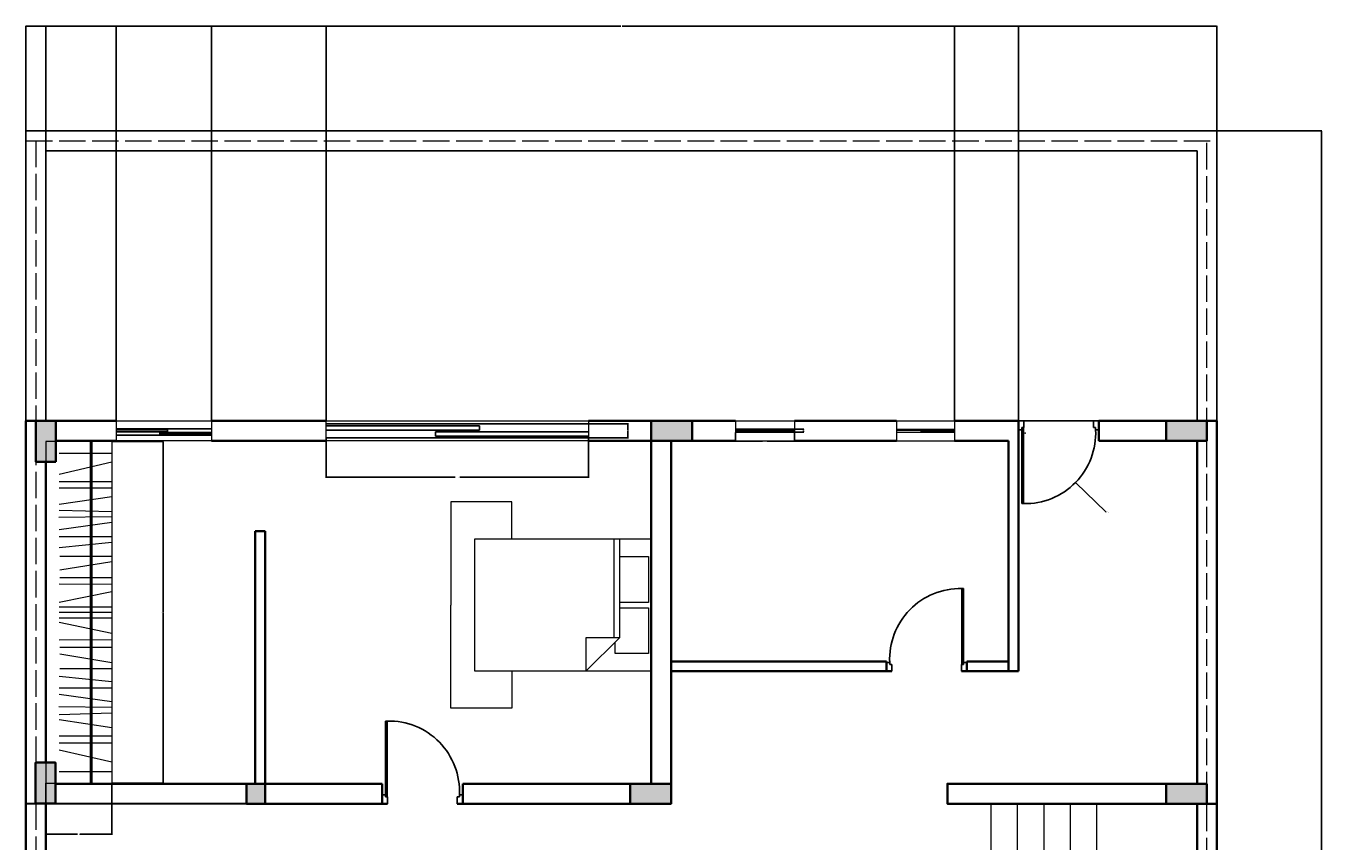
# Model space of a CAD drawing. Units: inches. Extents: x 2711 to 4246, y 540 to 1583.
# Tile 7 of 7: x 3658 to 4246, y 1213 to 1583. Entities that reach past the tile are written whole.
import ezdxf

# ---------------------------------------------------------------- set-up
doc = ezdxf.new("R2010")
doc.units = ezdxf.units.IN
doc.linetypes.add('ACAD_ISO02W100', pattern=[15, 12, -3])
for name, color, linetype, lineweight in [('A-ANNO-DIMS', 2, 'Continuous', 18), ('A-COLS', 210, 'Continuous', 35), ('A-COLS-PATT', 6, 'Continuous', 13), ('A-FLOR-CASE', 30, 'Continuous', 18), ('A-FLOR-STRS', 4, 'Continuous', 18), ('A-GLAZ', 4, 'Continuous', 18), ('A-WALL', 1, 'Continuous', 35), ('C-PROP-HIDN', 7, 'ACAD_ISO02W100', 13), ('C-PROP-WALL', 7, 'Continuous', 25), ('DOOR', 32, 'Continuous', 25), ('FURN', 30, 'Continuous', 18)]:
    doc.layers.add(name, color=color, linetype=linetype, lineweight=lineweight)
doc.layers.add('DARK', color=5, linetype='Continuous')
doc.styles.get("Standard").update_dxf_attribs({"font": 'arial.ttf'})
doc.dimstyles.get("Standard").update_dxf_attribs({"dimtxt": 0.18, "dimasz": 0.18, "dimexe": 0.18, "dimexo": 0.0625, "dimgap": 0.09, "dimtad": 0, "dimtih": 1, "dimtoh": 1, "dimdec": 4, "dimzin": 0, "dimdsep": 46, "dimtxsty": 'Standard', "dimcen": 0.09, "dimadec": 0, "dimazin": 0, "dimtfac": 1, "dimtdec": 4, "dimtofl": 0, "dimtmove": 0, "dimatfit": 3, "dimfxl": 1, "dimtolj": 1, "dimtzin": 0, "dimarcsym": 0})

# ---------------------------------------------------------------- blocks, each defined once
blk = doc.blocks.new('DOORS')
at = {"layer": 'DOOR'}
for p, q in [((-0.63, -0.36), (-0.63, -5.61)), ((-0.63, -5.61), (1.37, -5.61)), ((1.37, -5.61), (1.37, -4.36)), ((1.37, -4.36), (2.62, -4.36)), ((1.37, -5.61), (1.37, -49.61)), ((2.37, -49.61), (2.37, -4.36)), ((2.62, -4.36), (2.62, -0.36)), ((44.12, -4.36), (44.12, -0.36)), ((45.37, -4.36), (44.12, -4.36)), ((47.37, -5.61), (45.37, -5.61)), ((47.37, -0.36), (47.37, -5.61)), ((1.37, -49.61), (2.37, -49.61))]:
    blk.add_line(p, q, dxfattribs=at)
for centre, radius, start, end in [((3.41, -7.61), 42.01, 268.5852, 2.73188), ((38.76, -4.99), 6.64, 354.60229, 5.39771)]:
    blk.add_arc(centre, radius, start, end, dxfattribs=at)
blk = doc.blocks.new('DIPDASS')
at = {"layer": 'DARK'}
for p, q in [((0, 0), (109, 0)), ((0, -7.3), (109, -7.3))]:
    blk.add_line(p, q, dxfattribs=at)
at = {"layer": 'DOOR'}
for points in [[(0, -1.2), (56.3, -1.2), (58.8, -1.2), (58.8, -3.2), (56.3, -3.2), (0, -3.2)], [(109, -6.2), (52.7, -6.2), (50.2, -6.2), (50.2, -4.2), (52.7, -4.2), (109, -4.2)]]:
    blk.add_lwpolyline(points, dxfattribs=at)
blk = doc.blocks.new('DODO')
at = {"layer": 'DARK'}
for p, q in [((-118.96, 0), (0, 0)), ((-118.96, -6.4), (0, -6.4))]:
    blk.add_line(p, q, dxfattribs=at)
at = {"layer": 'DOOR'}
for p, q in [((-118.96, -0.88), (-49.49, -0.88)), ((-49.49, -2.88), (-118.96, -2.88)), ((0, -3.61), (-69.47, -3.61)), ((-69.47, -3.61), (-69.47, -5.61)), ((-69.47, -5.61), (0, -5.61)), ((-49.49, -0.88), (-49.49, -2.88))]:
    blk.add_line(p, q, dxfattribs=at)
blk = doc.blocks.new('Bed - Queen')
for p, q in [((0, -80.00003), (0, 0)), ((0, 0), (59.99999, 0)), ((59.99999, 0), (59.99999, -80.00003)), ((7.99999, -1.2), (28.79998, -1.2)), ((7.99999, -14.4), (7.99999, -1.2)), ((28.79998, -1.2), (28.79998, -14.4)), ((31.19999, -1.2), (51.99999, -1.2)), ((31.19999, -14.4), (31.19999, -1.2)), ((51.99999, -1.2), (51.99999, -16.4)), ((0, -14.4), (44.8, -14.4)), ((44.8, -16.8), (0, -16.8)), ((59.99999, -29.6), (44.8, -14.4)), ((44.8, -14.4), (44.8, -29.6)), ((51.99999, -16.4), (46.79936, -16.4)), ((44.8, -29.6), (59.99999, -29.6)), ((59.99999, -80.00003), (0, -80.00003))]:
    blk.add_line(p, q)
blk = doc.blocks.new('WARDROBE-LONG')
for p, q in [((29.95, 154.87), (0, 154.87)), ((0, 154.87), (0, 0)), ((20.07, 154.87), (20.07, 0)), ((20.11, 154.87), (20.11, 0)), ((20.16, 154.87), (20.16, 0)), ((20.2, 154.87), (20.2, 0)), ((20.23, 154.87), (20.23, 0)), ((20.29, 154.87), (20.29, 0)), ((20.35, 154.87), (20.35, 0)), ((20.41, 154.87), (20.41, 0)), ((20.45, 154.87), (20.45, 0)), ((20.49, 154.87), (20.49, 0)), ((20.55, 154.87), (20.55, 0)), ((20.6, 154.87), (20.6, 0)), ((20.66, 154.87), (20.66, 0)), ((20.73, 154.87), (20.73, 0)), ((20.78, 154.87), (20.78, 0)), ((20.83, 154.87), (20.83, 0)), ((20.87, 154.87), (20.87, 0)), ((20.92, 154.87), (20.92, 0)), ((20.92, 154.87), (20.92, 0)), ((29.95, 154.87), (29.95, 0)), ((6.03, 149.59), (29.95, 149.59)), ((29.95, 145.48), (6.03, 139.93)), ((6.03, 136.69), (29.95, 136.69)), ((29.95, 133.62), (6.03, 133.62)), ((29.95, 129.81), (6.03, 126.19)), ((6.03, 123.74), (29.95, 123.04)), ((29.95, 120.68), (5.93, 120.34)), ((29.95, 118.08), (6.01, 114.81)), ((6.01, 111.74), (29.95, 111.74)), ((29.95, 108.99), (6.01, 106.55)), ((6.38, 102.89), (29.95, 102.89)), ((29.95, 100.33), (6.38, 96.45)), ((29.95, 90.01), (6.01, 90.1)), ((6.38, 93.23), (29.95, 93.23)), ((6.01, 81.93), (29.95, 86.88)), ((6.01, 79.93), (29.95, 79.93)), ((6.01, 77.44), (29.95, 77.44)), ((6.01, 74.94), (29.95, 74.94)), ((6.01, 72.94), (29.95, 67.99)), ((29.95, 64.86), (6.01, 64.77)), ((6.38, 61.64), (29.95, 61.64)), ((29.95, 54.54), (6.38, 58.42)), ((29.95, 45.88), (6.01, 48.32)), ((6.38, 51.98), (29.95, 51.98)), ((6.01, 43.13), (29.95, 43.13)), ((29.95, 36.79), (6.01, 40.06)), ((29.95, 34.19), (5.93, 34.54)), ((6.03, 31.13), (29.95, 31.83)), ((29.95, 25.06), (6.03, 28.68)), ((29.95, 21.25), (6.03, 21.25)), ((6.03, 18.18), (29.95, 18.18)), ((29.95, 9.39), (6.03, 14.94)), ((0, 0), (29.95, 0)), ((6.03, 5.28), (29.95, 5.28))]:
    blk.add_line(p, q)
blk = doc.blocks.new('STAIR-RETURN')
for p, q in [((6.2, 174.01), (6.2, 138.01)), ((18.2, 174.01), (18.2, 138.01)), ((30.2, 174.01), (30.2, 138.01)), ((42.2, 174.01), (42.2, 138.01)), ((54.2, 174.01), (54.2, 138.01)), ((55.04, 138.01), (0, 138.01)), ((0, 138.01), (0, 135.01)), ((55.04, 133.05), (55.04, 138.01)), ((52.04, 135.01), (0, 135.01)), ((52.04, 39.5), (52.04, 135.01)), ((99.72, 133.05), (55.04, 133.05)), ((55.04, 37.05), (55.04, 133.05)), ((99.72, 121.05), (55.04, 121.05)), ((99.72, 109.05), (55.04, 109.05)), ((99.72, 97.05), (55.04, 97.05)), ((99.72, 85.05), (55.04, 85.05)), ((99.72, 73.05), (55.04, 73.05)), ((99.72, 61.05), (55.04, 61.05)), ((99.72, 49.05), (55.04, 49.05)), ((0, 36.5), (0, 39.5)), ((0, 39.5), (52.04, 39.5)), ((0, 36.5), (52.73, 36.5)), ((4.73, 36.5), (4.74, 0)), ((16.73, 36.5), (16.74, 0)), ((28.73, 36.5), (28.74, 0)), ((40.73, 36.5), (40.74, 0)), ((52.73, 36.5), (52.74, 0)), ((52.73, 36.5), (55.04, 36.5)), ((99.72, 37.05), (55.04, 37.05)), ((55.04, 36.5), (55.04, 37.05))]:
    blk.add_line(p, q)
blk = doc.blocks.new('WIN-SLIDER-W01')
for p, q in [((0, 9), (26.39, 9)), ((0, 9), (0, 0)), ((26.39, 9), (26.39, 0)), ((0, 5.31), (26.39, 5.31)), ((0, 5.11), (15.65, 5.11)), ((15.65, 4.66), (0, 4.66)), ((0, 3.87), (26.39, 3.87)), ((0, 0), (26.39, 0)), ((26.39, 4.5), (11.15, 4.5)), ((11.15, 4.5), (11.15, 4.05)), ((11.15, 4.05), (26.39, 4.05)), ((15.65, 5.11), (15.65, 4.66))]:
    blk.add_line(p, q)
blk = doc.blocks.new('BED-BASE-QUEEN')
for p, q in [((27.64, 93.59), (0, 93.59)), ((0, 93.59), (0, 46.79)), ((27.64, 76.79), (27.64, 93.59)), ((0, 0), (0, 46.79)), ((27.64, 16.79), (27.64, 0)), ((27.64, 0), (0, 0))]:
    blk.add_line(p, q)
blk = doc.blocks.new('*D66')
at = {"layer": 'A-ANNO-DIMS', "color": 0, "lineweight": -2, "transparency": 16777216}
for p, q in [((3794.34, 1395.69), (3794.34, 1377.73)), ((3913.3, 1395.69), (3913.3, 1377.73)), ((3794.52, 1377.91), (3852.73, 1377.91)), ((3913.12, 1377.91), (3854.9, 1377.91))]:
    blk.add_line(p, q, dxfattribs=at)
at = {"layer": 'A-ANNO-DIMS', "color": 0, "transparency": 16777216}
for points in [[(3794.52, 1377.94), (3794.52, 1377.88), (3794.34, 1377.91)], [(3913.12, 1377.94), (3913.12, 1377.88), (3913.3, 1377.91)]]:
    blk.add_solid(points, dxfattribs=at)
at = {"layer": 'Defpoints', "color": 0, "transparency": 16777216}
for p in [(3794.34, 1395.75), (3913.3, 1395.75), (3913.3, 1377.91)]:
    blk.add_point(p, dxfattribs=at)
at = {"layer": 'A-ANNO-DIMS', "color": 0, "transparency": 16777216, "insert": (3853.82, 1377.91), "char_height": 0.18, "attachment_point": 5}
blk.add_mtext('\\A1;SLIDER 119 TYP.', dxfattribs=at)
blk = doc.blocks.new('*D67')
at = {"layer": 'A-ANNO-DIMS', "color": 0, "lineweight": -2, "transparency": 16777216}
for p, q in [((3913.36, 1402.15), (3931.32, 1402.15)), ((3931.14, 1401.97), (3931.14, 1399.13)), ((3931.14, 1395.93), (3931.14, 1398.77)), ((3913.36, 1395.75), (3931.32, 1395.75))]:
    blk.add_line(p, q, dxfattribs=at)
at = {"layer": 'A-ANNO-DIMS', "color": 0, "transparency": 16777216}
for points in [[(3931.11, 1401.97), (3931.17, 1401.97), (3931.14, 1402.15)], [(3931.11, 1395.93), (3931.17, 1395.93), (3931.14, 1395.75)]]:
    blk.add_solid(points, dxfattribs=at)
at = {"layer": 'Defpoints', "color": 0, "transparency": 16777216}
for p in [(3913.3, 1402.15), (3931.14, 1402.15), (3913.3, 1395.75)]:
    blk.add_point(p, dxfattribs=at)
at = {"layer": 'A-ANNO-DIMS', "color": 0, "transparency": 16777216, "insert": (3931.14, 1398.95), "char_height": 0.18, "attachment_point": 5}
blk.add_mtext('\\A1;6 TYP.', dxfattribs=at)
blk = doc.blocks.new('*D68')
at = {"layer": 'A-ANNO-DIMS', "color": 0, "lineweight": -2, "transparency": 16777216}
for p, q in [((3979.84, 1398.26), (3979.84, 1394.12)), ((3980.02, 1394.3), (3992.22, 1394.3)), ((4006.46, 1394.3), (3994.26, 1394.3)), ((4006.64, 1398.26), (4006.64, 1394.12))]:
    blk.add_line(p, q, dxfattribs=at)
at = {"layer": 'A-ANNO-DIMS', "color": 0, "transparency": 16777216}
for points in [[(3980.02, 1394.33), (3980.02, 1394.27), (3979.84, 1394.3)], [(4006.46, 1394.33), (4006.46, 1394.27), (4006.64, 1394.3)]]:
    blk.add_solid(points, dxfattribs=at)
at = {"layer": 'Defpoints', "color": 0, "transparency": 16777216}
for p in [(3979.84, 1398.32), (4006.64, 1398.32), (4006.64, 1394.3)]:
    blk.add_point(p, dxfattribs=at)
at = {"layer": 'A-ANNO-DIMS', "color": 0, "transparency": 16777216, "insert": (3993.24, 1394.3), "char_height": 0.18, "attachment_point": 5}
blk.add_mtext('\\A1;SLIDER 27 TYP.', dxfattribs=at)
blk = doc.blocks.new('*D69')
at = {"layer": 'A-ANNO-DIMS', "color": 0, "lineweight": -2, "transparency": 16777216}
for p, q in [((4006.71, 1399.76), (4010.85, 1399.76)), ((4010.67, 1399.58), (4010.67, 1399.22)), ((4010.67, 1398.5), (4010.67, 1398.86)), ((4006.71, 1398.32), (4010.85, 1398.32))]:
    blk.add_line(p, q, dxfattribs=at)
at = {"layer": 'A-ANNO-DIMS', "color": 0, "transparency": 16777216}
for points in [[(4010.64, 1399.58), (4010.7, 1399.58), (4010.67, 1399.76)], [(4010.64, 1398.5), (4010.7, 1398.5), (4010.67, 1398.32)]]:
    blk.add_solid(points, dxfattribs=at)
at = {"layer": 'Defpoints', "color": 0, "transparency": 16777216}
for p in [(4006.64, 1399.76), (4010.67, 1399.76), (4006.64, 1398.32)]:
    blk.add_point(p, dxfattribs=at)
at = {"layer": 'A-ANNO-DIMS', "color": 0, "transparency": 16777216, "insert": (4010.67, 1399.04), "char_height": 0.18, "attachment_point": 5}
blk.add_mtext('\\A1;1 TYP.', dxfattribs=at)
blk = doc.blocks.new('*D80')
at = {"layer": 'A-ANNO-DIMS', "color": 0, "lineweight": -2, "transparency": 16777216}
for p, q in [((3697.2, 1394.18), (3720.55, 1394.18)), ((3720.37, 1394), (3720.37, 1316.93)), ((3720.37, 1239.49), (3720.37, 1316.56)), ((3697.2, 1239.31), (3720.55, 1239.31))]:
    blk.add_line(p, q, dxfattribs=at)
at = {"layer": 'A-ANNO-DIMS', "color": 0, "transparency": 16777216}
for points in [[(3720.34, 1394), (3720.4, 1394), (3720.37, 1394.18)], [(3720.34, 1239.49), (3720.4, 1239.49), (3720.37, 1239.31)]]:
    blk.add_solid(points, dxfattribs=at)
at = {"layer": 'Defpoints', "color": 0, "transparency": 16777216}
for p in [(3697.14, 1394.18), (3720.37, 1394.18), (3697.14, 1239.31)]:
    blk.add_point(p, dxfattribs=at)
at = {"layer": 'A-ANNO-DIMS', "color": 0, "transparency": 16777216, "insert": (3720.37, 1316.74), "char_height": 0.18, "attachment_point": 5}
blk.add_mtext('\\A1;WARDROBE 155 TYP.', dxfattribs=at)
blk = doc.blocks.new('*D81')
at = {"layer": 'A-ANNO-DIMS', "color": 0, "lineweight": -2, "transparency": 16777216}
for p, q in [((3667.18, 1239.24), (3667.18, 1215.9)), ((3697.14, 1239.24), (3697.14, 1215.9)), ((3667.36, 1216.08), (3681.63, 1216.08)), ((3696.96, 1216.08), (3682.69, 1216.08))]:
    blk.add_line(p, q, dxfattribs=at)
at = {"layer": 'A-ANNO-DIMS', "color": 0, "transparency": 16777216}
for points in [[(3667.36, 1216.11), (3667.36, 1216.05), (3667.18, 1216.08)], [(3696.96, 1216.11), (3696.96, 1216.05), (3697.14, 1216.08)]]:
    blk.add_solid(points, dxfattribs=at)
at = {"layer": 'Defpoints', "color": 0, "transparency": 16777216}
for p in [(3667.18, 1239.31), (3697.14, 1239.31), (3697.14, 1216.08)]:
    blk.add_point(p, dxfattribs=at)
at = {"layer": 'A-ANNO-DIMS', "color": 0, "transparency": 16777216, "insert": (3682.16, 1216.08), "char_height": 0.18, "attachment_point": 5}
blk.add_mtext('\\A1;30 TYP.', dxfattribs=at)
blk = doc.blocks.new('*D96')
at = {"layer": 'A-ANNO-DIMS', "color": 0, "lineweight": -2, "transparency": 16777216}
for p, q in [((3658.18, 1535.01), (3658.18, 1582.51)), ((3658.36, 1582.33), (3927.89, 1582.33)), ((4198, 1582.33), (3928.47, 1582.33)), ((4198.18, 1535.01), (4198.18, 1582.51))]:
    blk.add_line(p, q, dxfattribs=at)
at = {"layer": 'A-ANNO-DIMS', "color": 0, "transparency": 16777216}
for points in [[(3658.36, 1582.36), (3658.36, 1582.3), (3658.18, 1582.33)], [(4198, 1582.36), (4198, 1582.3), (4198.18, 1582.33)]]:
    blk.add_solid(points, dxfattribs=at)
at = {"layer": 'Defpoints', "color": 0, "transparency": 16777216}
for p in [(4198.18, 1582.33), (3658.18, 1534.95), (4198.18, 1534.95)]:
    blk.add_point(p, dxfattribs=at)
at = {"layer": 'A-ANNO-DIMS', "color": 0, "transparency": 16777216, "insert": (3928.18, 1582.33), "char_height": 0.18, "attachment_point": 5}
blk.add_mtext('\\A1;540', dxfattribs=at)
blk = doc.blocks.new('*D97')
at = {"layer": 'A-ANNO-DIMS', "color": 0, "lineweight": -2, "transparency": 16777216}
for p, q in [((4198.24, 1534.95), (4245.74, 1534.95)), ((4245.56, 1534.77), (4245.56, 1061.38)), ((4245.56, 587.63), (4245.56, 1061.02)), ((4198.24, 587.45), (4245.74, 587.45))]:
    blk.add_line(p, q, dxfattribs=at)
at = {"layer": 'A-ANNO-DIMS', "color": 0, "transparency": 16777216}
for points in [[(4245.53, 1534.77), (4245.59, 1534.77), (4245.56, 1534.95)], [(4245.53, 587.63), (4245.59, 587.63), (4245.56, 587.45)]]:
    blk.add_solid(points, dxfattribs=at)
at = {"layer": 'Defpoints', "color": 0, "transparency": 16777216}
for p in [(4198.18, 1534.95), (4245.56, 1534.95), (4198.18, 587.45)]:
    blk.add_point(p, dxfattribs=at)
at = {"layer": 'A-ANNO-DIMS', "color": 0, "transparency": 16777216, "insert": (4245.56, 1061.2), "char_height": 0.18, "attachment_point": 5}
blk.add_mtext('\\A1;947.5', dxfattribs=at)
blk = doc.blocks.new('*D116')
at = {"layer": 'A-ANNO-DIMS', "color": 0, "lineweight": -2, "transparency": 16777216}
for p, q in [((3667.18, 1403.51), (3667.18, 1582.51)), ((3667.36, 1582.33), (3682.73, 1582.33)), ((3698.88, 1582.33), (3683.52, 1582.33)), ((3699.06, 1403.51), (3699.06, 1582.51))]:
    blk.add_line(p, q, dxfattribs=at)
at = {"layer": 'A-ANNO-DIMS', "color": 0, "transparency": 16777216}
for points in [[(3667.36, 1582.36), (3667.36, 1582.3), (3667.18, 1582.33)], [(3698.88, 1582.36), (3698.88, 1582.3), (3699.06, 1582.33)]]:
    blk.add_solid(points, dxfattribs=at)
at = {"layer": 'Defpoints', "color": 0, "transparency": 16777216}
for p in [(3699.06, 1582.33), (3667.18, 1403.45), (3699.06, 1403.45)]:
    blk.add_point(p, dxfattribs=at)
at = {"layer": 'A-ANNO-DIMS', "color": 0, "transparency": 16777216, "insert": (3683.12, 1582.33), "char_height": 0.18, "attachment_point": 5}
blk.add_mtext('\\A1;31.88', dxfattribs=at)
blk = doc.blocks.new('*D117')
at = {"layer": 'A-ANNO-DIMS', "color": 0, "lineweight": -2, "transparency": 16777216}
for p, q in [((3742.3, 1403.51), (3742.3, 1582.51)), ((3742.48, 1582.33), (3767.93, 1582.33)), ((3794.16, 1582.33), (3768.71, 1582.33)), ((3794.34, 1403.51), (3794.34, 1582.51))]:
    blk.add_line(p, q, dxfattribs=at)
at = {"layer": 'A-ANNO-DIMS', "color": 0, "transparency": 16777216}
for points in [[(3742.48, 1582.36), (3742.48, 1582.3), (3742.3, 1582.33)], [(3794.16, 1582.36), (3794.16, 1582.3), (3794.34, 1582.33)]]:
    blk.add_solid(points, dxfattribs=at)
at = {"layer": 'Defpoints', "color": 0, "transparency": 16777216}
for p in [(3794.34, 1582.33), (3742.3, 1403.45), (3794.34, 1403.45)]:
    blk.add_point(p, dxfattribs=at)
at = {"layer": 'A-ANNO-DIMS', "color": 0, "transparency": 16777216, "insert": (3768.32, 1582.33), "char_height": 0.18, "attachment_point": 5}
blk.add_mtext('\\A1;52.04', dxfattribs=at)
blk = doc.blocks.new('*D119')
at = {"layer": 'A-ANNO-DIMS', "color": 0, "lineweight": -2, "transparency": 16777216}
for p, q in [((4079.23, 1403.51), (4079.23, 1582.51)), ((4079.41, 1582.33), (4093.24, 1582.33)), ((4108, 1582.33), (4094.17, 1582.33)), ((4108.18, 1403.51), (4108.18, 1582.51))]:
    blk.add_line(p, q, dxfattribs=at)
at = {"layer": 'A-ANNO-DIMS', "color": 0, "transparency": 16777216}
for points in [[(4079.41, 1582.36), (4079.41, 1582.3), (4079.23, 1582.33)], [(4108, 1582.36), (4108, 1582.3), (4108.18, 1582.33)]]:
    blk.add_solid(points, dxfattribs=at)
at = {"layer": 'Defpoints', "color": 0, "transparency": 16777216}
for p in [(4108.18, 1582.33), (4079.23, 1403.45), (4108.18, 1403.45)]:
    blk.add_point(p, dxfattribs=at)
at = {"layer": 'A-ANNO-DIMS', "color": 0, "transparency": 16777216, "insert": (4093.7, 1582.33), "char_height": 0.18, "attachment_point": 5}
blk.add_mtext('\\A1;28.954', dxfattribs=at)
blk = doc.blocks.new('*D131')
at = {"layer": 'A-ANNO-DIMS', "color": 0, "lineweight": -2, "transparency": 16777216}
for p, q in [((4111.16, 1397.93), (4111.34, 1397.93)), ((4111.25, 1397.84), (4111.25, 1398.02)), ((4147.83, 1362.18), (4134.24, 1375.46)), ((4148.01, 1362.18), (4147.83, 1362.18))]:
    blk.add_line(p, q, dxfattribs=at)
at = {"layer": 'A-ANNO-DIMS', "color": 0, "transparency": 16777216}
blk.add_solid([(4134.27, 1375.48), (4134.22, 1375.44), (4134.12, 1375.59)], dxfattribs=at)
at = {"layer": 'Defpoints', "color": 0, "transparency": 16777216}
for p in [(4111.25, 1397.93), (4134.12, 1375.59)]:
    blk.add_point(p, dxfattribs=at)
at = {"layer": 'A-ANNO-DIMS', "color": 0, "transparency": 16777216, "insert": (4148.69, 1362.18), "char_height": 0.18, "attachment_point": 5}
blk.add_mtext('\\A1;2X R31.97', dxfattribs=at)

msp = doc.modelspace()

# ---------------------------------------------------------------- hatches: boundary and pattern name
at = {"layer": 'A-COLS-PATT'}
h = msp.add_hatch(color=256, dxfattribs=at)
h.dxf.hatch_style = 1
h.paths.add_polyline_path([(3662.6812, 1384.9055), (3671.6812, 1384.9055), (3671.6812, 1403.4493), (3662.6812, 1403.4493)])
h.paths.add_polyline_path([(3960.225, 1394.4493), (3960.225, 1403.4493), (3941.6812, 1403.4493), (3941.6812, 1394.4493)])
h.paths.add_polyline_path([(4193.6812, 1394.4493), (4193.6812, 1403.4493), (4175.1375, 1403.4493), (4175.1375, 1394.4493)])
h.paths.add_polyline_path([(3662.5342, 1230.0438), (3671.5342, 1230.0353), (3671.5342, 1248.5791), (3662.5342, 1248.5791)])
h.paths.add_polyline_path([(3766.6812, 1229.9493), (3766.6812, 1238.9493), (3758.128, 1238.9493), (3758.128, 1229.9531), (3762.1812, 1229.9493)])
h.paths.add_polyline_path([(3950.6812, 1229.9493), (3950.6812, 1238.9493), (3932.1375, 1238.9493), (3932.1375, 1229.9493)])
h.paths.add_polyline_path([(4193.6812, 1229.9493), (4193.6812, 1238.9493), (4175.1375, 1238.9493), (4175.1375, 1229.9493)])
h.paths.add_polyline_path([(3671.5342, 1056.0394), (3662.5342, 1056.0394), (3662.5342, 1037.4957), (3671.5342, 1037.4957)])
h.paths.add_polyline_path([(3867.7072, 1041.7894), (3867.7072, 1037.4957), (3876.7006, 1037.4957), (3876.7006, 1056.0394), (3867.7006, 1056.0394), (3867.7006, 1052.2894), (3867.7072, 1052.2894), (3867.7072, 1047.0394)])
h.paths.add_polyline_path([(3957.7072, 1037.4957), (3957.7072, 1056.0394), (3948.7072, 1056.0394), (3948.7072, 1037.4957)])
h.paths.add_polyline_path([(4189.1812, 1046.9493), (4193.6812, 1046.9493), (4193.6812, 1055.9413), (4175.1375, 1055.9413), (4175.1375, 1046.9493)])
h.paths.add_polyline_path([(3876.7072, 924.0394), (3867.7072, 924.0394), (3867.7072, 905.4957), (3876.7072, 905.4957)])
h.paths.add_polyline_path([(3948.7072, 905.4957), (3957.7072, 905.4957), (3957.7072, 924.0394), (3948.7072, 924.0394)])
h.paths.add_polyline_path([(4110.7072, 905.7675), (4110.7072, 914.7675), (4092.1634, 914.7675), (4092.1634, 905.7675)])
h.paths.add_polyline_path([(3671.5342, 842.8947), (3671.5342, 861.4385), (3662.5342, 861.4385), (3662.5342, 842.8947)])
h.paths.add_polyline_path([(4189.1812, 824.7675), (4193.6812, 824.7498), (4193.6812, 833.7498), (4175.1375, 833.7498), (4175.1375, 824.7675)])
h.paths.add_polyline_path([(3688.2903, 587.4493), (3688.2903, 599.3563), (3662.6812, 599.3563), (3662.6812, 587.4493)])
h.paths.add_polyline_path([(3816.8435, 587.4493), (3816.8435, 596.4493), (3808.2903, 596.4493), (3808.2903, 587.4493)])
h.paths.add_polyline_path([(3890.4526, 587.4493), (3890.4526, 599.3563), (3864.8435, 599.3563), (3864.8435, 587.4493)])

# ---------------------------------------------------------------- linework, layer by layer
at = {"layer": 'A-COLS'}
for points in [[(3671.6812, 1384.9055), (3671.6812, 1403.4493), (3662.6812, 1403.4493), (3662.6812, 1384.9055)], [(3960.225, 1403.4493), (3941.6812, 1403.4493), (3941.6812, 1394.4493), (3960.225, 1394.4493)], [(4193.6812, 1403.4493), (4175.1375, 1403.4493), (4175.1375, 1394.4493), (4193.6812, 1394.4493)], [(3671.5342, 1230.0353), (3671.5342, 1248.5791), (3662.5342, 1248.5791), (3662.5342, 1230.0353)], [(3758.128, 1229.9493), (3766.6812, 1229.9493), (3766.6812, 1238.9493), (3758.128, 1238.9493)], [(3950.6812, 1238.9493), (3932.1375, 1238.9493), (3932.1375, 1229.9493), (3950.6812, 1229.9493)], [(4193.6812, 1238.9493), (4175.1375, 1238.9493), (4175.1375, 1229.9493), (4193.6812, 1229.9493)]]:
    msp.add_lwpolyline(points, close=True, dxfattribs=at)
at = {"layer": 'A-GLAZ'}
for p, q in [((3699.0637, 1403.4493), (3699.0637, 1394.4493)), ((3699.0637, 1403.4493), (3742.2997, 1403.4493)), ((3742.2997, 1403.4493), (3742.2997, 1394.4493)), ((3794.338, 1394.4493), (3794.338, 1403.4493)), ((3794.338, 1403.4493), (3913.2982, 1403.4493)), ((3913.2982, 1403.4493), (3913.2982, 1394.4493)), ((3979.8367, 1403.4493), (3979.8367, 1394.4493)), ((3979.8367, 1403.4493), (4006.645, 1403.4493)), ((4006.645, 1403.4493), (4006.645, 1394.4493)), ((3742.2997, 1394.4493), (3699.0637, 1394.4493)), ((3913.2982, 1394.4493), (3794.338, 1394.4493)), ((3979.8367, 1394.4493), (4006.645, 1394.4493))]:
    msp.add_line(p, q, dxfattribs=at)
at = {"layer": 'A-WALL'}
for p, q in [((3699.0637, 1403.4493), (3658.1812, 1403.4493)), ((3658.1812, 1403.4493), (3658.1812, 1230.048)), ((3794.338, 1403.4493), (3742.2997, 1403.4493)), ((3941.6812, 1403.4493), (3913.2982, 1403.4493)), ((3950.6812, 1403.4493), (3941.6812, 1403.4493)), ((3941.6812, 1403.4493), (3941.6812, 1238.9493)), ((3979.8367, 1403.4493), (3950.6812, 1403.4493)), ((4052.8385, 1403.4493), (4006.645, 1403.4493)), ((4103.6812, 1403.4493), (4079.2273, 1403.4493)), ((4108.1812, 1403.4493), (4103.6812, 1403.4493)), ((4108.1812, 1403.4493), (4108.1812, 1294.4493)), ((4189.1812, 1403.4493), (4144.7066, 1403.4493)), ((4144.7066, 1403.4493), (4144.7066, 1394.4493)), ((4198.1812, 1403.4493), (4189.1812, 1403.4493)), ((4198.1812, 1229.9493), (4198.1812, 1403.4493)), ((3671.6812, 1394.4493), (3699.0637, 1394.4493)), ((3742.2997, 1394.4493), (3794.338, 1394.4493)), ((3751.2319, 1394.4493), (3794.338, 1394.4493)), ((3913.2982, 1394.4493), (3941.6812, 1394.4493)), ((3950.6812, 1394.4493), (3941.6812, 1394.4493)), ((3979.8367, 1394.4493), (3950.6812, 1394.4493)), ((3950.6812, 1394.4493), (3950.6812, 1289.9493)), ((4052.8385, 1394.4493), (4006.645, 1394.4493)), ((4103.6812, 1394.4493), (4079.2273, 1394.4493)), ((4103.6812, 1394.4493), (4103.6812, 1289.9493)), ((4144.7066, 1394.4493), (4189.1812, 1394.4493)), ((4189.1812, 1394.4493), (4189.1812, 1238.9493)), ((3667.1812, 1248.5791), (3667.1812, 1384.9055)), ((3667.1812, 1248.5791), (3667.1812, 1384.9055)), ((3762.1812, 1353.5477), (3762.1812, 1238.9493)), ((3766.6812, 1353.5477), (3762.1812, 1353.5477)), ((3766.6812, 1238.9493), (3766.6812, 1353.5477)), ((4048.3152, 1294.4493), (3950.6812, 1294.4493)), ((4048.3152, 1294.4493), (4048.3152, 1289.9493)), ((4103.6812, 1294.4493), (4084.8405, 1294.4493)), ((4084.8405, 1294.4493), (4084.8405, 1289.9493)), ((4103.6812, 1289.9493), (4103.6812, 1294.4493)), ((4108.1812, 1294.4493), (4108.1812, 1289.9493)), ((3950.6812, 1289.9493), (4050.7883, 1289.9493)), ((3950.6812, 1289.9493), (3950.6812, 1238.9493)), ((4082.3674, 1289.9493), (4108.1812, 1289.9493)), ((3762.1812, 1238.9493), (3671.5342, 1238.9493)), ((3762.1812, 1238.9493), (3766.6812, 1238.9493)), ((3819.7072, 1238.9493), (3766.6812, 1238.9493)), ((3819.7072, 1238.9493), (3819.7072, 1229.9493)), ((3950.6812, 1238.9493), (3856.2325, 1238.9493)), ((3856.2325, 1229.9493), (3856.2325, 1238.9493)), ((3950.6812, 1238.9493), (3950.6812, 1229.9493)), ((3658.1812, 1230.048), (3762.1812, 1229.9493)), ((3658.1812, 1047.0394), (3658.1812, 1230.048)), ((3667.1812, 1056.0394), (3667.1812, 1230.0394)), ((3667.1812, 1230.0394), (3667.1812, 1056.0394)), ((3822.1802, 1229.9493), (3762.1812, 1229.9493)), ((3950.6812, 1229.9493), (3853.7594, 1229.9493)), ((4189.1812, 1229.9493), (4189.1812, 1055.9413)), ((4189.1812, 1229.9493), (4189.1812, 1055.9493)), ((4193.6812, 1229.9493), (4198.1812, 1229.9493)), ((4198.1812, 1046.9493), (4198.1812, 1229.9493))]:
    msp.add_line(p, q, dxfattribs=at)
msp.add_lwpolyline([(4189.1812, 1238.9493), (4108.1812, 1238.9493), (4075.9745, 1238.9493), (4075.9745, 1229.9493), (4108.1812, 1229.9493), (4189.1812, 1229.9493)], dxfattribs=at)
at = {"layer": 'C-PROP-HIDN'}
for p, q in [((3658.1812, 1530.4493), (4198.1812, 1530.4493)), ((3662.6812, 1530.4493), (3662.6812, 1248.5791)), ((4193.6812, 587.4493), (4193.6812, 1530.4493)), ((3662.6812, 1230.0353), (3662.6812, 1056.0394))]:
    msp.add_line(p, q, dxfattribs=at)
at = {"layer": 'C-PROP-WALL'}
for p, q in [((3658.1812, 1534.9493), (3662.6812, 1534.9493)), ((3658.1812, 1530.4493), (3658.1812, 1534.9493)), ((3662.6812, 1534.9493), (4193.6812, 1534.9493)), ((4193.6812, 1534.9493), (4198.1812, 1534.9493)), ((4198.1812, 1534.9493), (4198.1812, 1530.4493)), ((3658.1812, 587.4493), (3658.1812, 1530.4493)), ((4198.1812, 1530.4493), (4198.1812, 587.4493)), ((3667.1812, 1525.9493), (4189.1812, 1525.9493)), ((3667.1812, 1403.4493), (3667.1812, 1525.9493)), ((4189.1812, 1525.9493), (4189.1812, 1403.4493))]:
    msp.add_line(p, q, dxfattribs=at)
at = {"layer": 'DOOR'}
msp.add_line((4108.1812, 1403.4493), (4144.7066, 1403.4493), dxfattribs=at)

# ---------------------------------------------------------------- block references
at = {"layer": 'A-FLOR-CASE'}
msp.add_blockref('WARDROBE-LONG', (3667.1808, 1239.307), dxfattribs=at)
at = {"layer": 'A-FLOR-STRS'}
msp.add_blockref('STAIR-RETURN', (4089.4598, 1055.942), dxfattribs=at)
at = {"layer": 'A-GLAZ'}
for name, p, xscale, yscale, zscale in [('DIPDASS', (3699.0637, 1399.8345), 0.3965780416186425, 0.3965780416186425, 0.3965780416186425), ('DODO', (4006.645, 1399.7619), 0.2253547321596577, 0.2253547321596577, 0.2253547321596577)]:
    msp.add_blockref(name, p, dxfattribs=dict(at, xscale=xscale, yscale=yscale, zscale=zscale))
for name, p in [('DODO', (3913.2982, 1402.1484)), ('WIN-SLIDER-W01', (4052.8388, 1394.449))]:
    msp.add_blockref(name, p, dxfattribs=at)
at = {"layer": 'DOOR', "xscale": 0.7609445437706661, "yscale": 0.7609445437706661, "zscale": 0.7609445437706661}
msp.add_blockref('DOORS', (4108.6584, 1403.7248), dxfattribs=at)
at = {"layer": 'DOOR', "yscale": 0.7609445437706661, "zscale": 0.7609445437706661, "rotation": 180}
for p, xscale in [((4084.3634, 1289.6738), 0.7609445437706661), ((3820.1843, 1229.6738), -0.7609445437706661)]:
    msp.add_blockref('DOORS', p, dxfattribs=dict(at, xscale=xscale))
at = {"layer": 'FURN'}
msp.add_blockref('BED-BASE-QUEEN', (3850.8518, 1273.205), dxfattribs=at)
at = {"layer": 'FURN', "rotation": 270}
msp.add_blockref('Bed - Queen', (3941.6812, 1349.9992), dxfattribs=at)

# ---------------------------------------------------------------- dimensions: what is measured, and where the dimension line sits
at = {"layer": 'A-ANNO-DIMS'}
for base, p1, p2, override, picture, middle in [((4198.1812, 1582.3263), (3658.1812, 1534.9493), (4198.1812, 1534.9493), {"dimdec": 0, "dimlfac": 1, "dimrnd": 0, "dimzin": 0, "dimdsep": 46, "dimlunit": 2}, '*D96', (3928.1812, 1582.3263)), ((3699.0637, 1582.3263), (3667.1812, 1403.4493), (3699.0637, 1403.4493), {"dimdec": 2, "dimlfac": 1, "dimrnd": 0, "dimzin": 0, "dimdsep": 46, "dimlunit": 2}, '*D116', (3683.1224, 1582.3263)), ((3794.338, 1582.3263), (3742.2997, 1403.4493), (3794.338, 1403.4493), {"dimdec": 2, "dimlfac": 1, "dimrnd": 0, "dimzin": 0, "dimdsep": 46, "dimlunit": 2}, '*D117', (3768.3188, 1582.3263)), ((4108.1812, 1582.3263), (4079.2273, 1403.4493), (4108.1812, 1403.4493), {"dimdec": 3, "dimlfac": 1, "dimrnd": 0, "dimzin": 0, "dimdsep": 46, "dimlunit": 2}, '*D119', (4093.7043, 1582.3263))]:
    dim = msp.add_linear_dim(base=base, p1=p1, p2=p2, dimstyle='Standard', override=override, dxfattribs=at)
    dim.commit()
    dim.dimension.update_dxf_attribs({"geometry": picture, "text_midpoint": middle})
dim = msp.add_linear_dim(base=(4245.5582, 1534.9493), p1=(4198.1812, 587.4493), p2=(4198.1812, 1534.9493), angle=90, dimstyle='Standard', override={"dimdec": 1, "dimlfac": 1, "dimrnd": 0, "dimzin": 0, "dimdsep": 46, "dimlunit": 2}, dxfattribs=at)
dim.commit()
dim.dimension.update_dxf_attribs({"geometry": '*D97', "text_midpoint": (4245.5582, 1061.1993)})
for base, p1, p2, text, picture, middle in [((3931.1423, 1402.1484), (3913.2982, 1395.7502), (3913.2982, 1402.1484), '<> TYP.', '*D67', (3931.1423, 1398.9493)), ((4010.6662, 1399.7619), (4006.645, 1398.32), (4006.645, 1399.7619), '<> TYP.', '*D69', (4010.6662, 1399.041)), ((3720.3656, 1394.1774), (3697.1351, 1239.3071), (3697.1351, 1394.1774), 'WARDROBE <> TYP.', '*D80', (3720.3656, 1316.7423))]:
    dim = msp.add_linear_dim(base=base, p1=p1, p2=p2, angle=90, text=text, dimstyle='Standard', override={"dimdec": 0, "dimlfac": 1, "dimrnd": 0, "dimzin": 0, "dimdsep": 46, "dimlunit": 2}, dxfattribs=at)
    dim.commit()
    dim.dimension.update_dxf_attribs({"geometry": picture, "text_midpoint": middle})
for base, p1, p2, text, picture, middle in [((3913.2982, 1377.9061), (3794.338, 1395.7502), (3913.2982, 1395.7502), 'SLIDER <> TYP.', '*D66', (3853.8181, 1377.9061)), ((4006.645, 1394.2988), (3979.8367, 1398.32), (4006.645, 1398.32), 'SLIDER <> TYP.', '*D68', (3993.2408, 1394.2988)), ((3697.1351, 1216.0766), (3667.1812, 1239.3071), (3697.1351, 1239.3071), '<> TYP.', '*D81', (3682.1581, 1216.0766))]:
    dim = msp.add_linear_dim(base=base, p1=p1, p2=p2, text=text, dimstyle='Standard', override={"dimdec": 0, "dimlfac": 1, "dimrnd": 0, "dimzin": 0, "dimdsep": 46, "dimlunit": 2}, dxfattribs=at)
    dim.commit()
    dim.dimension.update_dxf_attribs({"geometry": picture, "text_midpoint": middle})
dim = msp.add_radius_dim(center=(4111.2534, 1397.9307), mpoint=(4134.1159, 1375.5871), text='2X <>', dimstyle='Standard', override={"dimdec": 2, "dimlfac": 1, "dimrnd": 0, "dimzin": 0, "dimdsep": 46, "dimlunit": 2}, dxfattribs=at)
dim.commit()
dim.dimension.update_dxf_attribs({"geometry": '*D131', "text_midpoint": (4148.6882, 1362.181), "dimtype": 164})

doc.saveas('drawing.dxf')
